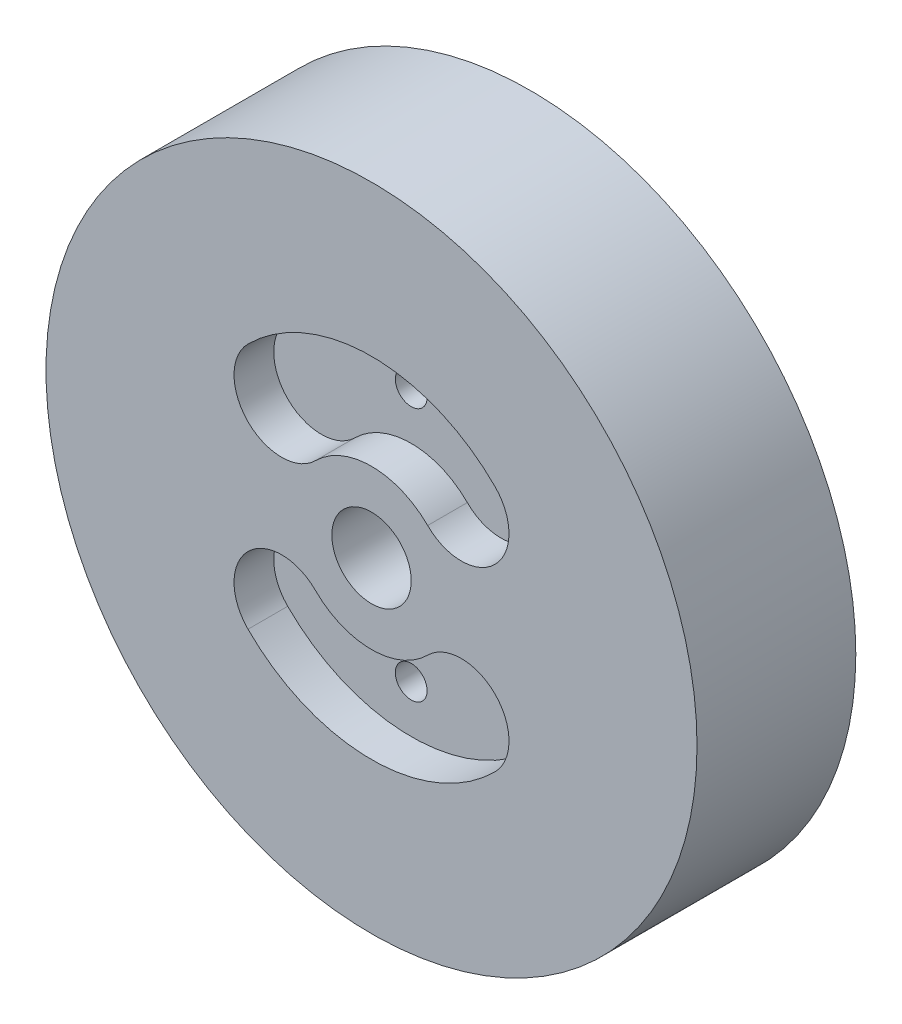
SolidWorks part; units mm, degrees
material "Plain Carbon Steel"
ref_plane "Front Plane" through (0, 0, 0) normal (0, 0, 1) x (1, 0, 0)
ref_plane "Top Plane" through (0, 0, 0) normal (0, 1, 0) x (1, 0, 0)
ref_plane "Right Plane" through (0, 0, 0) normal (1, 0, 0) x (0, 0, -1)
sketch "Disc Profile Ø41" plane through (0, 0, 0) normal (0, 0, 1) x (1, 0, 0)
  circle A0 centre (0, 0) radius 20.5
  dimension "D1" = 41
extrude "Port Block Disc" add sketch "Disc Profile Ø41" along normal blind 10
sketch "Arc Port Slots Profile" plane through (0, 0, 10) normal (0, 0, 1) x (1, 0, 0)
  arc A0 (7.7782, 7.7782) -> (-7.7782, 7.7782) centre (0, 0) ccw
  arc A1 (3.5355, 3.5355) -> (-3.5355, 3.5355) centre (0, 0) ccw
  circle A2 centre (0, 0) radius 8 construction
  arc A3 (3.5355, 3.5355) -> (7.7782, 7.7782) centre (5.6569, 5.6569) ccw
  arc A4 (-3.5355, 3.5355) -> (-7.7782, 7.7782) centre (-5.6569, 5.6569) cw
  arc A5 (3.5355, -3.5355) -> (-3.5355, -3.5355) centre (0, 0) cw
  arc A6 (-3.5355, -3.5355) -> (-7.7782, -7.7782) centre (-5.6569, -5.6569) ccw
  arc A7 (7.7782, -7.7782) -> (-7.7782, -7.7782) centre (0, 0) cw
  arc A8 (3.5355, -3.5355) -> (7.7782, -7.7782) centre (5.6569, -5.6569) cw
  dimension "D1" = 11
  dimension "D2" = 5
  dimension "D3" = 11
  dimension "D4" = 5
  dimension "D5" = 3
  dimension "D6" = 3
  dimension "D7" = 3
  dimension "D8" = 3
  dimension "D9" = 5.6569
  dimension "D10" = 5.6569
  dimension "D11" = 5.6569
  dimension "D12" = 5.6569
  dimension "D13" = 7.7782
  dimension "D14" = 7.7782
extrude "Arc Port Slots" cut sketch "Arc Port Slots Profile" against normal blind 2.5
sketch "Through Ports Profile" plane through (0, 0, 10) normal (0, 0, 1) x (1, 0, 0)
  circle A0 centre (0, 0) radius 2.5
  circle A1 centre (0, 0) radius 8 construction
  circle A2 centre (0, 8) radius 1
  circle A3 centre (0, -8) radius 1
  dimension "D1" = 2
  dimension "D2" = 2
  dimension "D3" = 5
extrude "Through Ports" cut sketch "Through Ports Profile" against normal blind 32.5
sketch "Port Pockets Profile" plane through (0, 0, 0) normal (0, 0, -1) x (-1, 0, 0)
  circle A0 centre (12.5, 0) radius 2.5
  circle A1 centre (-12.5, 0) radius 2.5
  dimension "D1" = 5
  dimension "D2" = 5
  dimension "D3" = 12.5
  dimension "D4" = 12.5
extrude "Port Pockets" cut sketch "Port Pockets Profile" against normal blind 5
